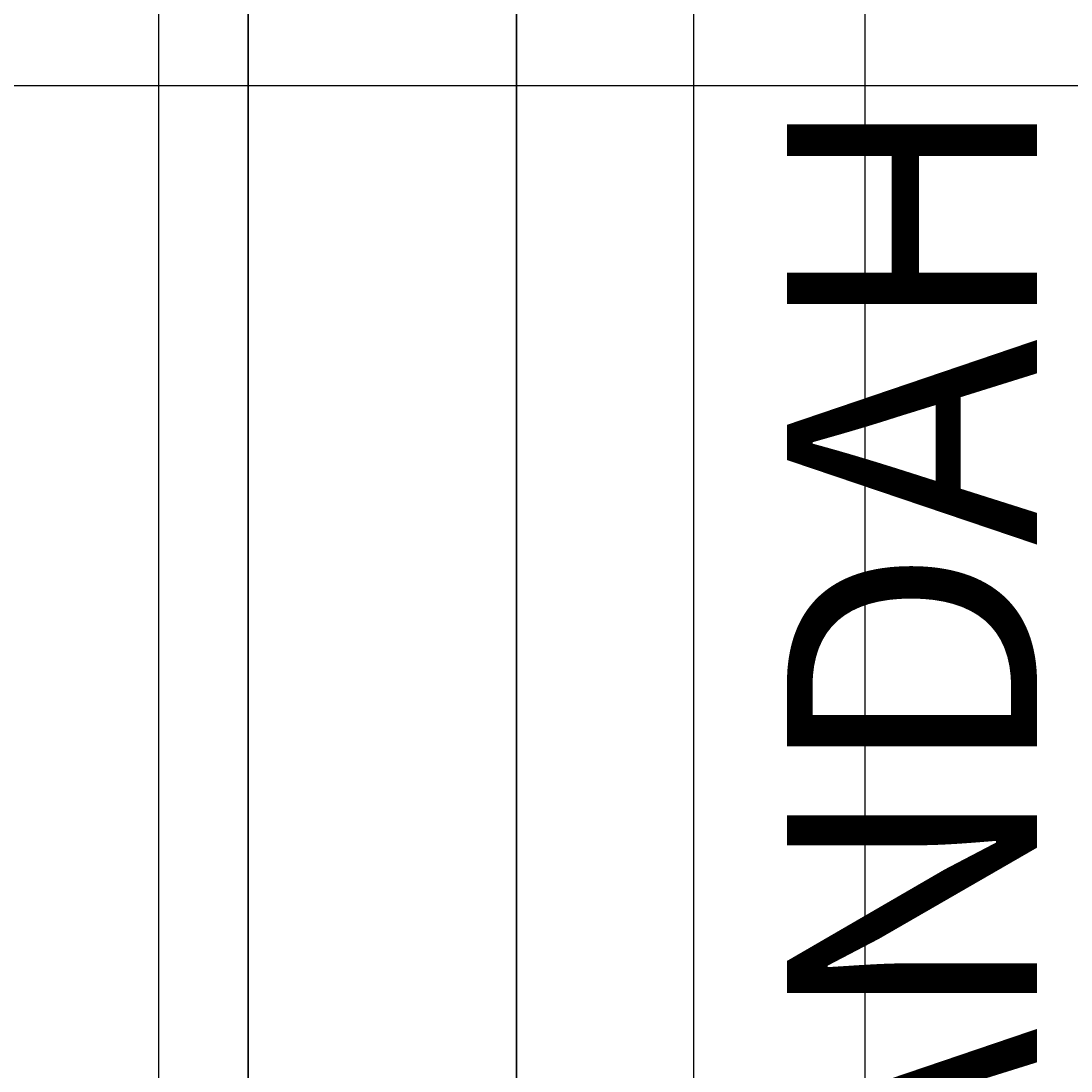
# Model space of a CAD drawing. Units: feet. Extents: x 1654 to 2985, y 1348 to 2230.
# Tile 12 of 53: x 1991 to 2027, y 1608 to 1643. Entities that reach past the tile are written whole.
import ezdxf

# ---------------------------------------------------------------- set-up
doc = ezdxf.new("R2010")
doc.units = ezdxf.units.FT
for name, color, linetype, lineweight in [('A-ANNO-DIMS', 2, 'Continuous', 18), ('A-AREA-IDEN', 7, 'Continuous', 18), ('A-WALL', 7, 'Continuous', 35)]:
    doc.layers.add(name, color=color, linetype=linetype, lineweight=lineweight)
doc.styles.get("Standard").update_dxf_attribs({"font": 'arial.ttf'})
doc.dimstyles.get("Standard").update_dxf_attribs({"dimtxt": 0.18, "dimasz": 0.18, "dimexe": 0.18, "dimexo": 0.0625, "dimgap": 0.09, "dimtad": 0, "dimtih": 1, "dimtoh": 1, "dimdec": 4, "dimzin": 0, "dimdsep": 46, "dimtxsty": 'Standard', "dimcen": 0.09, "dimadec": 0, "dimazin": 0, "dimtfac": 1, "dimtdec": 4, "dimtofl": 0, "dimtmove": 0, "dimatfit": 3, "dimfxl": 1, "dimtolj": 1, "dimtzin": 0, "dimarcsym": 0})

# ---------------------------------------------------------------- blocks, each defined once
blk = doc.blocks.new('*D90')
at = {"layer": 'A-ANNO-DIMS', "color": 0, "lineweight": -2, "transparency": 16777216}
for p, q in [((1852.155, 1641.187), (2242.272, 1641.187)), ((2242.092, 1641.007), (2242.092, 1607.903)), ((2242.092, 1574.435), (2242.092, 1607.539)), ((1852.155, 1574.255), (2242.272, 1574.255))]:
    blk.add_line(p, q, dxfattribs=at)
at = {"layer": 'A-ANNO-DIMS', "color": 0, "transparency": 16777216}
for points in [[(2242.062, 1641.007), (2242.122, 1641.007), (2242.092, 1641.187)], [(2242.062, 1574.435), (2242.122, 1574.435), (2242.092, 1574.255)]]:
    blk.add_solid(points, dxfattribs=at)
at = {"layer": 'Defpoints', "color": 0, "transparency": 16777216}
for p in [(1852.092, 1641.187), (2242.092, 1641.187), (1852.092, 1574.255)]:
    blk.add_point(p, dxfattribs=at)
at = {"layer": 'A-ANNO-DIMS', "color": 0, "transparency": 16777216, "insert": (2242.092, 1607.721), "char_height": 0.18, "attachment_point": 5}
blk.add_mtext('\\A1;66.93', dxfattribs=at)
blk = doc.blocks.new('*D101')
at = {"layer": 'A-ANNO-DIMS', "color": 0, "lineweight": -2, "transparency": 16777216}
for p, q in [((1996.092, 2039.192), (1996.092, 1534.075)), ((2014.016, 2039.192), (2014.016, 1534.075)), ((1996.272, 1534.255), (2004.599, 1534.255)), ((2013.836, 1534.255), (2005.509, 1534.255))]:
    blk.add_line(p, q, dxfattribs=at)
at = {"layer": 'A-ANNO-DIMS', "color": 0, "transparency": 16777216}
for points in [[(1996.272, 1534.285), (1996.272, 1534.225), (1996.092, 1534.255)], [(2013.836, 1534.285), (2013.836, 1534.225), (2014.016, 1534.255)]]:
    blk.add_solid(points, dxfattribs=at)
at = {"layer": 'Defpoints', "color": 0, "transparency": 16777216}
for p in [(1996.092, 2039.255), (2014.016, 2039.255), (2014.016, 1534.255)]:
    blk.add_point(p, dxfattribs=at)
at = {"layer": 'A-ANNO-DIMS', "color": 0, "transparency": 16777216, "insert": (2005.054, 1534.255), "char_height": 0.18, "attachment_point": 5}
blk.add_mtext('\\A1;17.924', dxfattribs=at)
blk = doc.blocks.new('*D102')
at = {"layer": 'A-ANNO-DIMS', "color": 0, "lineweight": -2, "transparency": 16777216}
for p, q in [((2008.092, 1742.192), (2008.092, 1534.075)), ((2019.757, 1742.192), (2019.757, 1534.075)), ((2008.272, 1534.255), (2013.47, 1534.255)), ((2019.577, 1534.255), (2014.379, 1534.255))]:
    blk.add_line(p, q, dxfattribs=at)
at = {"layer": 'A-ANNO-DIMS', "color": 0, "transparency": 16777216}
for points in [[(2008.272, 1534.285), (2008.272, 1534.225), (2008.092, 1534.255)], [(2019.577, 1534.285), (2019.577, 1534.225), (2019.757, 1534.255)]]:
    blk.add_solid(points, dxfattribs=at)
at = {"layer": 'Defpoints', "color": 0, "transparency": 16777216}
for p in [(2008.092, 1742.255), (2019.757, 1742.255), (2019.757, 1534.255)]:
    blk.add_point(p, dxfattribs=at)
at = {"layer": 'A-ANNO-DIMS', "color": 0, "transparency": 16777216, "insert": (2013.925, 1534.255), "char_height": 0.18, "attachment_point": 5}
blk.add_mtext('\\A1;11.664', dxfattribs=at)

msp = doc.modelspace()

# ---------------------------------------------------------------- linework, layer by layer
at = {"layer": 'A-WALL'}
for p, q in [((1999.0924, 1600.2549), (1999.0924, 1742.2549)), ((2008.0924, 1600.2549), (2008.0924, 1661.2549))]:
    msp.add_line(p, q, dxfattribs=at)

# ---------------------------------------------------------------- texts
at = {"layer": 'A-AREA-IDEN'}
msp.add_text('VERANDAH', height=8.38114, rotation=90, dxfattribs=at).set_placement((2025.5306, 1582.1049))

# ---------------------------------------------------------------- dimensions: what is measured, and where the dimension line sits
at = {"layer": 'A-ANNO-DIMS'}
for base, p1, p2, picture, middle in [((2014.016, 1534.2549), (1996.0924, 2039.2549), (2014.016, 2039.2549), '*D101', (2005.0542, 1534.2549)), ((2019.7567, 1534.2549), (2008.0924, 1742.2549), (2019.7567, 1742.2549), '*D102', (2013.9246, 1534.2549))]:
    dim = msp.add_linear_dim(base=base, p1=p1, p2=p2, dimstyle='Standard', override={"dimdec": 3, "dimlfac": 1, "dimrnd": 0, "dimzin": 0, "dimdsep": 46, "dimlunit": 2}, dxfattribs=at)
    dim.commit()
    dim.dimension.update_dxf_attribs({"geometry": picture, "text_midpoint": middle})
dim = msp.add_linear_dim(base=(2242.0924, 1641.187), p1=(1852.0924, 1574.2549), p2=(1852.0924, 1641.187), angle=90, dimstyle='Standard', override={"dimdec": 2, "dimlfac": 1, "dimrnd": 0, "dimzin": 0, "dimdsep": 46, "dimlunit": 2}, dxfattribs=at)
dim.commit()
dim.dimension.update_dxf_attribs({"geometry": '*D90', "text_midpoint": (2242.0924, 1607.721)})

doc.saveas('drawing.dxf')
